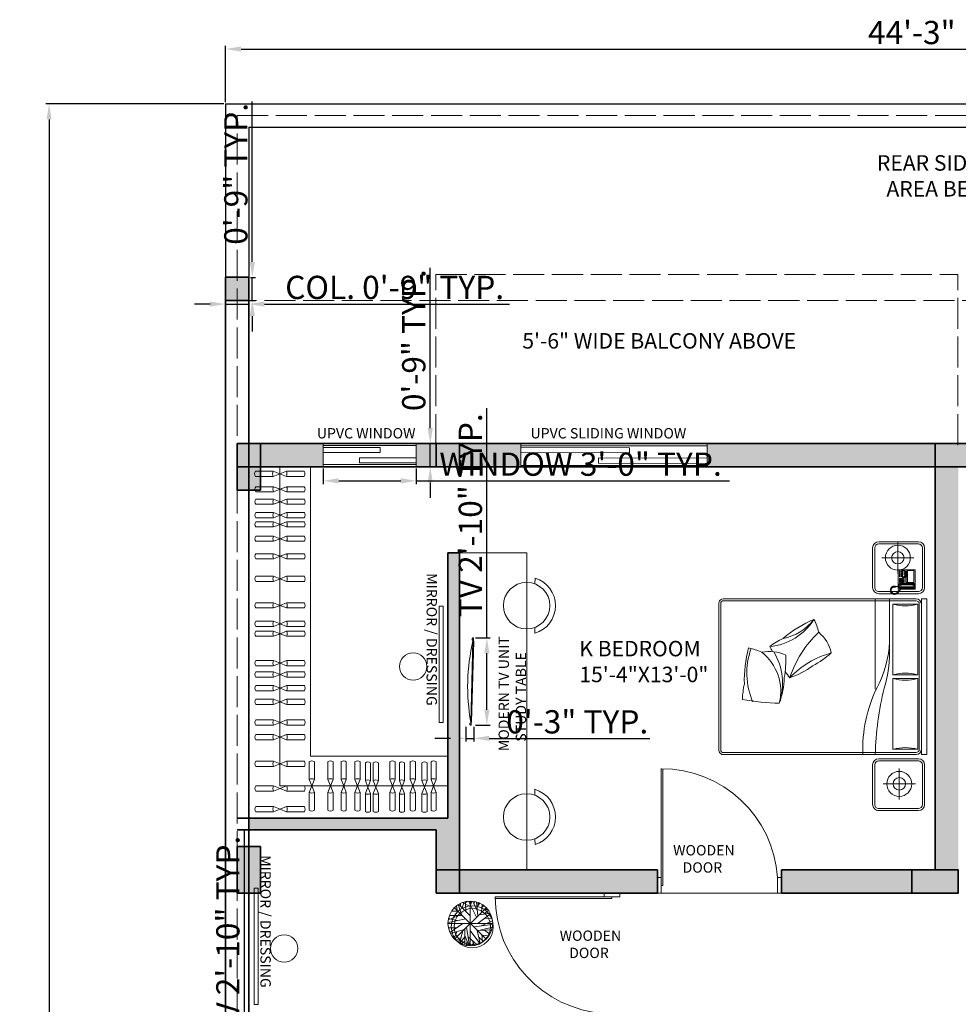
# Model space of a CAD drawing. Units: millimetres. Extents: x 595116 to 630915, y 909473 to 920225.
# Tile 133 of 134: x 630214 to 630577, y 919741 to 920122. Entities that reach past the tile are written whole.
import ezdxf

# ---------------------------------------------------------------- set-up
doc = ezdxf.new("R2010")
doc.units = ezdxf.units.MM
doc.linetypes.add('ACAD_ISO02W100', pattern=[15, 12, -3])
for name, color, linetype, lineweight in [('A-AREA-IDEN', 7, 'Continuous', 20), ('A-EQPM', 8, 'Continuous', 13), ('A-FLOR-BALC', 152, 'Continuous', 18), ('A-FLOR-OVHD', 253, 'ACAD_ISO02W100', 13), ('A-FURN', 32, 'Continuous', 18), ('A-WALL', 1, 'Continuous', 35), ('A-WALL-PATT', 8, 'Continuous', 13), ('C-PROP', 7, 'Continuous', 25), ('C-PROP-REF', 240, 'ACAD_ISO02W100', 13), ('Column', 6, 'Continuous', 35), ('Dimension', 3, 'Continuous', 18), ('Doors', 31, 'Continuous', 20), ('L-PLNT', 85, 'Continuous', 13), ('Text', 7, 'Continuous', 18), ('Windows', 33, 'Continuous', 18)]:
    doc.layers.add(name, color=color, linetype=linetype, lineweight=lineweight)
doc.styles.get("Standard").update_dxf_attribs({"font": 'arial.ttf'})
doc.dimstyles.new('ISO-25', dxfattribs={"dimtxt": 9, "dimasz": 6, "dimexe": 1.25, "dimexo": 0.625, "dimtad": 1, "dimlunit": 4, "dimtxsty": 'Standard', "dimcen": 2.5, "dimadec": 0, "dimazin": 0, "dimtfac": 1, "dimtmove": 0, "dimatfit": 3, "dimfxl": 1, "dimarcsym": 0})

# ---------------------------------------------------------------- blocks, each defined once
blk = doc.blocks.new('KWD')
for points in [[(629753.63, 919957.93), (629752.54, 919957.93), (629752.54, 919953.43), (629753.63, 919953.43)], [(629787.45, 919957.93), (629787.45, 919953.43), (629788.54, 919953.43), (629788.54, 919957.93)]]:
    blk.add_lwpolyline(points, close=True)
blk.add_lwpolyline([(629753.63, 919921.79), (629753.63, 919955.68), (629754.13, 919955.68), (629754.13, 919921.8)])
blk.add_arc((629753.64, 919955.68), 33.88, 269.99, 356.196)
blk = doc.blocks.new('A$C356F0359')
for p, q in [((0.5489, 2), (2.0492, 2)), ((0.5489, 1.9489), (0.5489, 2)), ((2.0492, 1.9489), (2.0492, 2)), ((-0.0002, 1.9201), (-0.0002, 1.5401)), ((0.0198, 1.9201), (0.0198, 1.5401)), ((0.4398, 1.9801), (0.0598, 1.9801)), ((0.4398, 1.9601), (0.0598, 1.9601)), ((0.4798, 1.5401), (0.4798, 1.9201)), ((0.4998, 1.5401), (0.4998, 1.9201)), ((2.0492, 1.9489), (0.5489, 1.9489)), ((0.5489, 1.8977), (0.5489, 0.0512)), ((0.5689, 1.8977), (0.5689, 0.0512)), ((1.998, 1.9289), (0.6001, 1.9289)), ((2.0292, 0.0512), (2.0292, 1.8977)), ((2.0492, 0.0512), (2.0492, 1.8977)), ((2.0883, 1.9201), (2.0883, 1.5401)), ((2.1083, 1.9201), (2.1083, 1.5401)), ((2.5283, 1.9801), (2.1483, 1.9801)), ((2.5283, 1.9601), (2.1483, 1.9601)), ((2.5683, 1.5401), (2.5683, 1.9201)), ((2.5883, 1.5401), (2.5883, 1.9201)), ((0.1539, 1.5681), (0.1539, 1.8777)), ((0.2725, 1.8879), (0.2702, 1.8856)), ((0.2702, 1.8856), (0.2702, 1.7279)), ((0.2725, 1.8879), (0.4531, 1.8879)), ((0.3913, 1.8753), (0.277, 1.8753)), ((0.277, 1.8753), (0.277, 1.8147)), ((0.277, 1.8147), (0.3913, 1.8147)), ((0.3913, 1.8125), (0.2816, 1.8125)), ((0.2816, 1.8125), (0.2816, 1.801)), ((0.2816, 1.801), (0.3913, 1.801)), ((0.2907, 1.8125), (0.2907, 1.801)), ((0.2999, 1.8125), (0.2999, 1.801)), ((0.309, 1.8125), (0.309, 1.801)), ((0.3182, 1.8125), (0.3182, 1.801)), ((0.3273, 1.8125), (0.3273, 1.801)), ((0.3365, 1.8125), (0.3365, 1.801)), ((0.3913, 1.8147), (0.3913, 1.8753)), ((0.3913, 1.801), (0.3913, 1.8125)), ((0.4016, 1.8787), (0.4062, 1.8845)), ((0.4016, 1.7404), (0.4016, 1.8787)), ((0.4062, 1.881), (0.405, 1.8765)), ((0.405, 1.8765), (0.4153, 1.8662)), ((0.405, 1.8765), (0.405, 1.8456)), ((0.405, 1.8456), (0.4073, 1.8399)), ((0.4062, 1.8845), (0.4405, 1.8845)), ((0.4108, 1.8833), (0.4062, 1.881)), ((0.4073, 1.8399), (0.4108, 1.8342)), ((0.4108, 1.8833), (0.4382, 1.8833)), ((0.4165, 1.8685), (0.4108, 1.8833)), ((0.4108, 1.8342), (0.4119, 1.8262)), ((0.4119, 1.8262), (0.4119, 1.8147)), ((0.4119, 1.793), (0.4119, 1.8147)), ((0.4153, 1.8662), (0.4165, 1.8685)), ((0.4153, 1.8147), (0.4153, 1.8662)), ((0.4153, 1.8147), (0.4153, 1.753)), ((0.4325, 1.8685), (0.4165, 1.8685)), ((0.4325, 1.8685), (0.4382, 1.8833)), ((0.4336, 1.8662), (0.4325, 1.8685)), ((0.4439, 1.8765), (0.4336, 1.8662)), ((0.4336, 1.8147), (0.4336, 1.8662)), ((0.4336, 1.8147), (0.4336, 1.753)), ((0.4382, 1.8342), (0.4371, 1.8262)), ((0.4371, 1.8262), (0.4371, 1.8147)), ((0.4371, 1.793), (0.4371, 1.8147)), ((0.4382, 1.8833), (0.4428, 1.881)), ((0.4416, 1.8399), (0.4382, 1.8342)), ((0.4405, 1.8845), (0.4462, 1.8787)), ((0.4439, 1.8456), (0.4416, 1.8399)), ((0.4428, 1.881), (0.4439, 1.8765)), ((0.4439, 1.8765), (0.4439, 1.8456)), ((0.4462, 1.8787), (0.4462, 1.7416)), ((0.4531, 1.8879), (0.4553, 1.8856)), ((0.4553, 1.8856), (0.4553, 1.7279)), ((2.3306, 1.5822), (2.3306, 1.8917)), ((0.3052, 1.7226), (0.0051, 1.7226)), ((0.2702, 1.7279), (0.2725, 1.7256)), ((0.4244, 1.7256), (0.2725, 1.7256)), ((0.277, 1.7885), (0.277, 1.7679)), ((0.3445, 1.7885), (0.277, 1.7885)), ((0.277, 1.7679), (0.3445, 1.7679)), ((0.2782, 1.7622), (0.2782, 1.7576)), ((0.2896, 1.7622), (0.2782, 1.7622)), ((0.2782, 1.7576), (0.2896, 1.7576)), ((0.2782, 1.745), (0.2896, 1.745)), ((0.2782, 1.7382), (0.2782, 1.745)), ((0.2896, 1.7382), (0.2782, 1.7382)), ((0.2885, 1.7862), (0.2885, 1.7827)), ((0.2919, 1.7862), (0.2885, 1.7862)), ((0.2885, 1.7827), (0.2919, 1.7827)), ((0.2919, 1.7736), (0.2885, 1.7736)), ((0.2885, 1.7736), (0.2885, 1.7702)), ((0.2885, 1.7702), (0.2919, 1.7702)), ((0.2896, 1.7576), (0.2896, 1.7622)), ((0.2896, 1.745), (0.2896, 1.7382)), ((0.2919, 1.7827), (0.2919, 1.7862)), ((0.2919, 1.7702), (0.2919, 1.7736)), ((0.2942, 1.7622), (0.2942, 1.7576)), ((0.3056, 1.7622), (0.2942, 1.7622)), ((0.2942, 1.7576), (0.3056, 1.7576)), ((0.2942, 1.745), (0.3056, 1.745)), ((0.2942, 1.7382), (0.2942, 1.745)), ((0.3056, 1.7382), (0.2942, 1.7382)), ((0.3056, 1.7576), (0.3056, 1.7622)), ((0.3056, 1.745), (0.3056, 1.7382)), ((0.3125, 1.7862), (0.309, 1.7862)), ((0.309, 1.7862), (0.309, 1.7827)), ((0.309, 1.7827), (0.3125, 1.7827)), ((0.3125, 1.7736), (0.309, 1.7736)), ((0.309, 1.7736), (0.309, 1.7702)), ((0.309, 1.7702), (0.3125, 1.7702)), ((0.3102, 1.7622), (0.3102, 1.7576)), ((0.3216, 1.7622), (0.3102, 1.7622)), ((0.3102, 1.7576), (0.3216, 1.7576)), ((0.3102, 1.745), (0.3216, 1.745)), ((0.3102, 1.7382), (0.3102, 1.745)), ((0.3216, 1.7382), (0.3102, 1.7382)), ((0.3125, 1.7827), (0.3125, 1.7862)), ((0.3125, 1.7702), (0.3125, 1.7736)), ((0.3216, 1.7576), (0.3216, 1.7622)), ((0.3216, 1.745), (0.3216, 1.7382)), ((0.3376, 1.7622), (0.3262, 1.7622)), ((0.3262, 1.7622), (0.3262, 1.7576)), ((0.3262, 1.7576), (0.3376, 1.7576)), ((0.3262, 1.7382), (0.3262, 1.745)), ((0.3262, 1.745), (0.3376, 1.745)), ((0.3376, 1.7382), (0.3262, 1.7382)), ((0.333, 1.7862), (0.3296, 1.7862)), ((0.3296, 1.7862), (0.3296, 1.7827)), ((0.3296, 1.7827), (0.333, 1.7827)), ((0.333, 1.7736), (0.3296, 1.7736)), ((0.3296, 1.7736), (0.3296, 1.7702)), ((0.3296, 1.7702), (0.333, 1.7702)), ((0.333, 1.7827), (0.333, 1.7862)), ((0.333, 1.7702), (0.333, 1.7736)), ((0.3376, 1.7576), (0.3376, 1.7622)), ((0.3376, 1.745), (0.3376, 1.7382)), ((0.3445, 1.7679), (0.3445, 1.7885)), ((0.3548, 1.7759), (0.3548, 1.7827)), ((0.3548, 1.7827), (0.3639, 1.7827)), ((0.3639, 1.7759), (0.3548, 1.7759)), ((0.3548, 1.7633), (0.3548, 1.7702)), ((0.3548, 1.7702), (0.3639, 1.7702)), ((0.3639, 1.7633), (0.3548, 1.7633)), ((0.3548, 1.7564), (0.3639, 1.7564)), ((0.3548, 1.7496), (0.3548, 1.7564)), ((0.3639, 1.7496), (0.3548, 1.7496)), ((0.3548, 1.737), (0.3548, 1.7439)), ((0.3548, 1.7439), (0.3639, 1.7439)), ((0.3639, 1.737), (0.3548, 1.737)), ((0.3639, 1.7827), (0.3639, 1.7759)), ((0.3639, 1.7702), (0.3639, 1.7633)), ((0.3639, 1.7564), (0.3639, 1.7496)), ((0.3639, 1.7439), (0.3639, 1.737)), ((0.3685, 1.7827), (0.3776, 1.7827)), ((0.3685, 1.7759), (0.3685, 1.7827)), ((0.3776, 1.7759), (0.3685, 1.7759)), ((0.3685, 1.7633), (0.3685, 1.7702)), ((0.3685, 1.7702), (0.3776, 1.7702)), ((0.3776, 1.7633), (0.3685, 1.7633)), ((0.3685, 1.7564), (0.3776, 1.7564)), ((0.3685, 1.7496), (0.3685, 1.7564)), ((0.3776, 1.7496), (0.3685, 1.7496)), ((0.3685, 1.737), (0.3685, 1.7439)), ((0.3685, 1.7439), (0.3776, 1.7439)), ((0.3776, 1.737), (0.3685, 1.737)), ((0.3776, 1.7827), (0.3776, 1.7759)), ((0.3776, 1.7702), (0.3776, 1.7633)), ((0.3776, 1.7564), (0.3776, 1.7496)), ((0.3776, 1.7439), (0.3776, 1.737)), ((0.3822, 1.7759), (0.3822, 1.7827)), ((0.3822, 1.7827), (0.3913, 1.7827)), ((0.3913, 1.7759), (0.3822, 1.7759)), ((0.3822, 1.7633), (0.3822, 1.7702)), ((0.3822, 1.7702), (0.3913, 1.7702)), ((0.3913, 1.7633), (0.3822, 1.7633)), ((0.3822, 1.7576), (0.3913, 1.7576)), ((0.3822, 1.7507), (0.3822, 1.7576)), ((0.3913, 1.7507), (0.3822, 1.7507)), ((0.3822, 1.7439), (0.3913, 1.7439)), ((0.3822, 1.737), (0.3822, 1.7439)), ((0.3913, 1.737), (0.3822, 1.737)), ((0.3913, 1.7827), (0.3913, 1.7759)), ((0.3913, 1.7702), (0.3913, 1.7633)), ((0.3913, 1.7576), (0.3913, 1.7507)), ((0.3913, 1.7439), (0.3913, 1.737)), ((0.4073, 1.7347), (0.4016, 1.7404)), ((0.405, 1.7736), (0.4073, 1.7793)), ((0.405, 1.7427), (0.405, 1.7736)), ((0.405, 1.7427), (0.4153, 1.753)), ((0.4062, 1.7382), (0.405, 1.7427)), ((0.4108, 1.7359), (0.4062, 1.7382)), ((0.4073, 1.7793), (0.4108, 1.785)), ((0.4234, 1.7347), (0.4073, 1.7347)), ((0.4108, 1.785), (0.4119, 1.793)), ((0.4165, 1.7507), (0.4108, 1.7359)), ((0.4108, 1.7359), (0.4234, 1.7359)), ((0.4153, 1.753), (0.4165, 1.7507)), ((0.4325, 1.7507), (0.4165, 1.7507)), ((0.4233, 1.7393), (0.4235, 1.7294)), ((0.4268, 1.7393), (0.4233, 1.7393)), ((0.4235, 1.7294), (0.4263, 1.7179)), ((0.4263, 1.7179), (0.429, 1.707)), ((0.4274, 1.7301), (0.4268, 1.7393)), ((0.427, 1.7359), (0.4382, 1.7359)), ((0.4405, 1.7347), (0.4271, 1.7347)), ((0.429, 1.7227), (0.4274, 1.7301)), ((0.4531, 1.7256), (0.4284, 1.7256)), ((0.429, 1.707), (0.4288, 1.701)), ((0.4318, 1.7119), (0.429, 1.7227)), ((0.4325, 1.7063), (0.4318, 1.7119)), ((0.4323, 1.7003), (0.4325, 1.7063)), ((0.4336, 1.753), (0.4325, 1.7507)), ((0.4325, 1.7507), (0.4382, 1.7359)), ((0.4439, 1.7427), (0.4336, 1.753)), ((0.4382, 1.785), (0.4371, 1.793)), ((0.4416, 1.7793), (0.4382, 1.785)), ((0.4382, 1.7359), (0.4428, 1.7382)), ((0.4462, 1.7416), (0.4405, 1.7347)), ((0.4439, 1.7736), (0.4416, 1.7793)), ((0.4428, 1.7382), (0.4439, 1.7427)), ((0.4439, 1.7427), (0.4439, 1.7736)), ((0.4553, 1.7279), (0.4531, 1.7256)), ((0.4622, 1.7459), (0.4553, 1.7484)), ((0.4553, 1.7439), (0.4604, 1.7425)), ((0.4604, 1.7425), (0.465, 1.7388)), ((0.4654, 1.7427), (0.4622, 1.7459)), ((0.465, 1.7388), (0.4662, 1.7372)), ((0.4678, 1.7405), (0.4654, 1.7427)), ((0.4662, 1.7372), (0.4686, 1.7374)), ((0.4686, 1.7374), (0.4662, 1.735)), ((0.4662, 1.735), (0.4755, 1.7268)), ((0.4721, 1.7421), (0.4678, 1.7405)), ((0.4741, 1.7401), (0.4721, 1.7421)), ((0.4725, 1.7366), (0.4741, 1.7401)), ((0.4753, 1.7388), (0.4725, 1.7366)), ((0.4783, 1.7356), (0.4753, 1.7388)), ((0.4755, 1.7268), (0.4906, 1.7139)), ((0.4759, 1.729), (0.4783, 1.7356)), ((0.4821, 1.7322), (0.4759, 1.729)), ((0.4874, 1.7272), (0.4821, 1.7322)), ((0.4862, 1.7199), (0.4874, 1.7272)), ((0.4914, 1.7231), (0.4862, 1.7199)), ((0.4908, 1.7135), (0.4984, 1.6917)), ((0.4958, 1.7185), (0.4914, 1.7231)), ((0.494, 1.7135), (0.4958, 1.7185)), ((0.501, 1.7142), (0.494, 1.7135)), ((0.4964, 1.7047), (0.5031, 1.7072)), ((0.5031, 1.7072), (0.501, 1.7142)), ((2.4819, 1.7366), (2.1818, 1.7366)), ((0.427, 1.697), (0.4265, 1.6915)), ((0.4265, 1.6915), (0.4332, 1.6903)), ((0.4332, 1.6903), (0.4267, 1.6864)), ((0.4267, 1.6864), (0.4272, 1.6801)), ((0.4295, 1.6996), (0.427, 1.697)), ((0.4272, 1.6801), (0.4346, 1.6794)), ((0.4346, 1.6794), (0.4281, 1.6744)), ((0.4281, 1.6744), (0.4311, 1.669)), ((0.4288, 1.701), (0.4295, 1.6996)), ((0.4311, 1.669), (0.4381, 1.6704)), ((0.4364, 1.6973), (0.4323, 1.7003)), ((0.4381, 1.6704), (0.4348, 1.6639)), ((0.4348, 1.6639), (0.4383, 1.6598)), ((0.4355, 1.6919), (0.4364, 1.6973)), ((0.4367, 1.6774), (0.4355, 1.6919)), ((0.4455, 1.6663), (0.4367, 1.6774)), ((0.4383, 1.6598), (0.4436, 1.6637)), ((0.4436, 1.6637), (0.4427, 1.6575)), ((0.4427, 1.6575), (0.4471, 1.6547)), ((0.4577, 1.6598), (0.4455, 1.6663)), ((0.4471, 1.6547), (0.4526, 1.6593)), ((0.4526, 1.6593), (0.4519, 1.6517)), ((0.4519, 1.6517), (0.4568, 1.6503)), ((0.4568, 1.6503), (0.4598, 1.6565)), ((0.4716, 1.6586), (0.4577, 1.6598)), ((0.4598, 1.6565), (0.4626, 1.6503)), ((0.4626, 1.6503), (0.4665, 1.6498)), ((0.4665, 1.6498), (0.4681, 1.6565)), ((0.4681, 1.6565), (0.4707, 1.6491)), ((0.4707, 1.6491), (0.4751, 1.6503)), ((0.485, 1.6644), (0.4716, 1.6586)), ((0.4751, 1.6503), (0.4753, 1.6565)), ((0.4753, 1.6565), (0.4806, 1.6519)), ((0.4806, 1.6519), (0.4843, 1.6538)), ((0.4843, 1.6538), (0.4836, 1.6607)), ((0.4836, 1.6607), (0.4885, 1.6547)), ((0.4952, 1.6744), (0.485, 1.6644)), ((0.4885, 1.6547), (0.4922, 1.6579)), ((0.4922, 1.6579), (0.4894, 1.6642)), ((0.4894, 1.6642), (0.4959, 1.6614)), ((0.4984, 1.6917), (0.4952, 1.6744)), ((0.4957, 1.6704), (0.5024, 1.6683)), ((0.4989, 1.6642), (0.4957, 1.6704)), ((0.4959, 1.6614), (0.4989, 1.6642)), ((0.5038, 1.7049), (0.4964, 1.7047)), ((0.5042, 1.673), (0.4987, 1.6792)), ((0.4987, 1.6792), (0.5058, 1.679)), ((0.5005, 1.695), (0.5054, 1.6996)), ((0.5068, 1.695), (0.5005, 1.695)), ((0.5008, 1.6871), (0.5079, 1.6892)), ((0.5068, 1.6836), (0.5008, 1.6871)), ((0.5024, 1.6683), (0.5042, 1.673)), ((0.5054, 1.6996), (0.5038, 1.7049)), ((0.5058, 1.679), (0.5068, 1.6836)), ((0.5079, 1.6892), (0.5068, 1.695)), ((0.0598, 1.5001), (0.4398, 1.5001)), ((0.0598, 1.4801), (0.4398, 1.4801)), ((2.1483, 1.5001), (2.5283, 1.5001)), ((2.1483, 1.4801), (2.5283, 1.4801)), ((0.6001, 0.02), (1.998, 0.02)), ((0.6001, 0), (1.998, 0))]:
    blk.add_line(p, q)
at = {"linetype": 'ByBlock'}
for p, q in [((0.6001, 1.9147), (1.282, 1.9147)), ((0.6001, 1.6759), (0.6001, 1.9147)), ((1.282, 1.9147), (1.282, 1.6759)), ((1.3161, 1.9147), (1.998, 1.9147)), ((1.3161, 1.6759), (1.3161, 1.9147)), ((1.998, 1.9147), (1.998, 1.6759)), ((1.0687, 1.6418), (0.5489, 1.6418)), ((1.282, 1.6759), (0.6001, 1.6759)), ((1.998, 1.6759), (1.3161, 1.6759)), ((1.4185, 1.5053), (0.5489, 1.5053))]:
    blk.add_line(p, q, dxfattribs=at)
for centre in [(0.1539, 1.7226), (2.3306, 1.7366)]:
    blk.add_circle(centre, 0.12, dxfattribs=at)
for centre in [(0.1539, 1.7226), (2.3306, 1.7366)]:
    blk.add_circle(centre, 0.06)
for centre, radius, start, end in [((0.0598, 1.9201), 0.06, 90, 180), ((0.0598, 1.9201), 0.04, 90, 180), ((0.4398, 1.9201), 0.06, 0, 90), ((0.4398, 1.9201), 0.04, 0, 90), ((0.6001, 1.8977), 0.0512, 90, 180), ((0.6001, 1.8977), 0.0312, 90, 180), ((1.998, 1.8977), 0.0512, 0, 90), ((1.998, 1.8977), 0.0312, 0, 90), ((2.1483, 1.9201), 0.06, 90, 180), ((2.1483, 1.9201), 0.04, 90, 180), ((2.5283, 1.9201), 0.06, 0, 90), ((2.5283, 1.9201), 0.04, 0, 90), ((0.0598, 1.5401), 0.06, 180, 270), ((0.0598, 1.5401), 0.04, 180, 270), ((0.4398, 1.5401), 0.04, 270, 0), ((0.4398, 1.5401), 0.06, 270, 0), ((2.1483, 1.5401), 0.06, 180, 270), ((2.1483, 1.5401), 0.04, 180, 270), ((2.5283, 1.5401), 0.06, 270, 0), ((2.5283, 1.5401), 0.04, 270, 0), ((1.1471, 0.7332), 0.3575, 102.47819, 140.46254), ((1.9086, 1.3124), 0.8697, 195.33601, 226.41927), ((0.3249, 0.4335), 0.9879, 28.49711, 41.05657), ((0.9965, 0.4273), 0.548, 103.20343, 117.03623), ((1.6529, 1.7059), 1.0798, 223.63057, 251.4288), ((0.4451, 0.4375), 0.5655, 5.33912, 57.68949), ((0.4517, 0.5274), 0.4879, 10.69865, 52.68638), ((1.8195, 1.3719), 1.1652, 203.06416, 220.32086), ((0.5617, 0.4344), 0.7874, 18.35266, 36.68512), ((-0.021, 2.4319), 2.1977, 305.29657, 307.24182), ((1.5949, 0.9312), 0.734, 205.25901, 216.93514), ((1.4135, 0.487), 0.3575, 154.0418, 192.02615), ((1.3641, 0.0041), 0.6085, 71.81005, 120.13512), ((1.44, 0.1186), 0.4774, 76.18494, 142.00166), ((1.1372, -0.3434), 0.9879, 80.06073, 92.62018), ((1.2836, -0.1573), 0.7874, 69.91627, 88.24873), ((-0.6432, 0.628), 2.1977, 349.48843, 358.80544), ((-0.021, 2.4319), 2.1977, 297.92482, 299.3793), ((1.5595, 0.1789), 0.548, 154.76704, 168.59984), ((1.3312, 1.4107), 1.1652, 254.62778, 271.88448), ((1.2647, 0.9578), 0.6885, 250.29361, 293.6414), ((1.5368, 0.9609), 0.734, 256.82263, 268.49876), ((0.5943, 0.0454), 0.0458, 172.75992, 277.24008), ((0.5943, 0.0454), 0.0258, 172.75992, 277.24008), ((2.0038, 0.0454), 0.0458, 262.75992, 7.24008), ((2.0038, 0.0454), 0.0258, 262.75992, 7.24008)]:
    blk.add_arc(centre, radius, start, end)
for centre, radius, start, end in [((0.1906, 1.7953), 0.4265, 343.73979, 16.26021), ((1.6914, 1.7953), 0.4265, 163.73979, 196.26021), ((0.9067, 1.7953), 0.4265, 343.73979, 16.26021), ((2.4075, 1.7953), 0.4265, 163.73979, 196.26021), ((0.9303, 0.657), 0.9853, 61.43285, 88.12613), ((1.0826, 0.5712), 1.0706, 72.19663, 90.74184), ((2.0056, 2.7745), 1.3903, 244.24266, 271.79845), ((2.1368, 4.5996), 3.0955, 256.42012, 268.37887)]:
    blk.add_arc(centre, radius, start, end, dxfattribs=at)
blk = doc.blocks.new('*D129')
at = {"layer": 'Defpoints', "color": 0, "transparency": 16777216}
for p in [(630824.6, 920110.68), (630293.6, 920089.43), (630824.6, 920089.43)]:
    blk.add_point(p, dxfattribs=at)
at = {"layer": 'Dimension', "color": 0, "lineweight": -2, "transparency": 16777216}
for p, q in [((630293.6, 920090.05), (630293.6, 920111.93)), ((630824.6, 920090.05), (630824.6, 920111.93)), ((630299.6, 920110.68), (630818.6, 920110.68))]:
    blk.add_line(p, q, dxfattribs=at)
at = {"layer": 'Dimension', "color": 0, "transparency": 16777216}
for points in [[(630299.6, 920111.68), (630299.6, 920109.68), (630293.6, 920110.68)], [(630818.6, 920111.68), (630818.6, 920109.68), (630824.6, 920110.68)]]:
    blk.add_solid(points, dxfattribs=at)
at = {"layer": 'Dimension', "color": 0, "transparency": 16777216, "insert": (630559.1, 920115.9), "char_height": 9, "attachment_point": 5}
blk.add_mtext('44\'-3"', dxfattribs=at)
blk = doc.blocks.new('TV-PLAN')
for p, q in [((2.04, 32.58), (1.21, 1.19)), ((2.14, 32.58), (1.31, 1.19)), ((2.24, 32.58), (1.41, 1.19)), ((2.34, 32.57), (1.51, 1.18)), ((2.04, 32.58), (2.34, 32.57)), ((2.14, 32.58), (2.14, 33.76)), ((2.19, 32.58), (2.19, 33.76)), ((1.21, 1.19), (1.51, 1.18)), ((1.31, 1.19), (1.31, 0.01)), ((1.36, 1.19), (1.36, 0.01))]:
    blk.add_line(p, q)
for centre, radius, start, end in [((76.63, 14.9), 76.65, 166.662, 190.3006), ((2.09, 33.31), 0.462, 77.1755, 282.8245), ((1.26, 0.46), 0.462, 77.1755, 282.8245)]:
    blk.add_arc(centre, radius, start, end)
blk = doc.blocks.new('WARDROBE-HANGER')
for p, q in [((9.73, 1), (9.73, 1)), ((9.73, 1), (12.27, 0)), ((9.73, 1), (9.73, 1)), ((12.27, 2), (19.15, 2)), ((0.32, 0), (7.19, 0)), ((12.27, 0), (19.15, 0))]:
    blk.add_line(p, q)
for points in [[(7.19, 2), (0.32, 2, 0.315389), (0.32, 0)], [(9.73, 1), (7.19, 2, 0.225748), (7.19, 0), (9.73, 1), (12.27, 2)]]:
    blk.add_lwpolyline(points, format="xyb")
for centre, radius, start, end in [((10.17, 1), 2.33, 334.5576, 25.4424), ((17.71, 1), 1.74, 324.9906, 35.0094)]:
    blk.add_arc(centre, radius, start, end)
blk = doc.blocks.new('POTTED-PLANT')
for p, q in [((14.75, 15.51), (2.6, 3.36)), ((14.75, 3.36), (2.6, 15.51)), ((2.87, 15.88), (3.4, 15.68)), ((3.32, 16.24), (3.58, 14.57)), ((3.96, 16.73), (5.31, 12.84)), ((4.16, 16.82), (8.64, 12.35)), ((4.85, 16.17), (4.88, 17.22)), ((5.49, 15.52), (6.28, 17.77)), ((5.61, 17.51), (8.67, 15.94)), ((6.86, 17.38), (7.52, 18.03)), ((6.89, 14.08), (6.86, 17.93)), ((7.9, 18.06), (11.06, 11.86)), ((9.02, 17.38), (8.46, 18.1)), ((8.67, 18.11), (8.67, 0.76)), ((8.74, 16.47), (9.2, 18.06)), ((11.32, 14.57), (9.46, 18.06)), ((10.09, 16.89), (10.53, 17.9)), ((11.52, 12.26), (11.04, 17.77)), ((11.14, 16.82), (12.03, 17.41)), ((11.24, 15.75), (12.36, 17.28)), ((13.25, 16.79), (13.05, 13.86)), ((13.17, 15.58), (13.86, 16.4)), ((4.01, 12.42), (0.12, 10.79)), ((0.57, 12.45), (5.66, 12.45)), ((1.47, 14.18), (3.93, 14.18)), ((16.53, 13.1), (11.7, 9.48)), ((12.05, 12.81), (16.38, 13.4)), ((13.91, 13.07), (15.74, 14.51)), ((14.04, 14.8), (15.41, 14.87)), ((0, 9.44), (17.35, 9.44)), ((0.04, 9.84), (6.94, 11.18)), ((0.19, 11.28), (3.48, 10.53)), ((0.22, 7.66), (3.4, 7.75)), ((0.78, 5.86), (5.74, 9.45)), ((7.22, 7.98), (8.31, 0.8)), ((10.02, 8.11), (17.3, 9.03)), ((12.49, 6.77), (17.19, 8.01)), ((12.92, 8.47), (17.27, 10.46)), ((14.24, 11.38), (17.09, 11.41)), ((0.98, 5.47), (6.25, 7.04)), ((3.99, 4.75), (1.72, 4.29)), ((3.48, 6.19), (2.31, 3.58)), ((5.1, 3.97), (3.07, 2.83)), ((5.79, 6.51), (4.54, 1.82)), ((6.56, 4.2), (4.67, 1.78)), ((6.53, 7.26), (6.56, 1.1)), ((6.56, 4.78), (8.11, 0.84)), ((7.78, 4.2), (11.26, 1.2)), ((8.67, 6.68), (12.41, 1.65)), ((11.37, 6.74), (12.54, 1.72)), ((11.39, 6.74), (16.97, 6.94)), ((11.98, 4.16), (13.78, 2.43)), ((13.07, 5.08), (13.35, 2.21)), ((13.22, 4.91), (15.85, 4.62)), ((14.19, 6.81), (16.25, 5.24)), ((4.88, 3.09), (3.65, 2.4)), ((6.56, 2.6), (5.05, 1.59)), ((5.56, 2.86), (5.79, 1.33)), ((7.45, 2.57), (7.01, 0.97)), ((7.75, 1.82), (7.32, 0.93)), ((9.89, 1.75), (9.23, 0.84)), ((9.53, 2.7), (10.2, 0.97)), ((12.26, 2.96), (12, 1.49))]:
    blk.add_line(p, q)
for centre, radius in [((8.67, 9.44), 8.67), ((9.43, 8.14), 8.14), ((9.43, 8.14), 7.03)]:
    blk.add_circle(centre, radius)
blk = doc.blocks.new('WIN-UPVC-3FT')
for p, q in [((0, 0), (0, 9)), ((0, 9), (36, 9)), ((36, 0), (36, 9)), ((0, 7.5), (22, 7.5)), ((0, 5.5), (22, 5.5)), ((22, 7.5), (22, 5.5)), ((14, 3.5), (36, 3.5)), ((14, 3.5), (14, 1.5)), ((14, 1.5), (36, 1.5)), ((0, 0), (36, 0))]:
    blk.add_line(p, q)
blk.add_lwpolyline([(0, 8.25), (36, 8.25), (36, 0.89), (0, 0.89)], close=True)
blk = doc.blocks.new('WIN-SLIDING-6FT')
for p, q in [((0, 0), (0, 9)), ((0, 9), (72, 9)), ((72, 0), (72, 9)), ((0, 5.5), (42, 5.41)), ((0.01, 7.5), (42, 7.41)), ((42, 7.41), (42, 5.41)), ((30, 3.44), (72, 3.35)), ((30, 3.44), (30, 1.44)), ((30, 1.44), (71.99, 1.35)), ((0, 0), (72, 0))]:
    blk.add_line(p, q)
blk.add_lwpolyline([(0, 8.12), (72, 8.12), (72, 0.59), (0, 0.59)], close=True)
blk = doc.blocks.new('CHAIR-ROUND')
for p, q in [((12.11, 21.41), (12.12, 19.12)), ((12.2, 2.29), (12.22, 0))]:
    blk.add_line(p, q)
blk.add_circle((8.99, 10.69), 8.99)
blk.add_arc((8.99, 10.69), 11.16, 286.7943, 73.7898)
blk = doc.blocks.new('COLUMN-SQUARE-9IN')
h = blk.add_hatch(color=256)
h.dxf.hatch_style = 1
h.paths.add_polyline_path([(9, 9), (0, 9), (0, 0), (9, 0)])
blk.add_lwpolyline([(0, 9), (9, 9), (9, 0), (0, 0)], close=True)
blk = doc.blocks.new('COLUMN-RECT-18X9')
h = blk.add_hatch(color=256)
h.dxf.hatch_style = 1
h.paths.add_polyline_path([(18, 9), (0, 9), (0, 0), (18, 0)])
blk.add_lwpolyline([(0, 9), (18, 9), (18, 0), (0, 0)], close=True)
blk = doc.blocks.new('COLUMN-RECT-9X18')
h = blk.add_hatch(color=256)
h.dxf.hatch_style = 1
h.paths.add_polyline_path([(9, 18), (0, 18), (0, 0), (9, 0)])
blk.add_lwpolyline([(0, 18), (9, 18), (9, 0), (0, 0)], close=True)
blk = doc.blocks.new('*D156')
at = {"layer": 'Defpoints', "color": 0, "transparency": 16777216}
for p in [(630293.6, 920013.3), (630302.6, 920013.3), (630302.6, 920011.95)]:
    blk.add_point(p, dxfattribs=at)
at = {"layer": 'Dimension', "color": 0, "lineweight": -2, "transparency": 16777216}
for p, q in [((630293.6, 920012.68), (630293.6, 920010.7)), ((630302.6, 920012.68), (630302.6, 920010.7)), ((630287.6, 920011.95), (630281.6, 920011.95)), ((630293.6, 920011.95), (630302.6, 920011.95)), ((630308.6, 920011.95), (630403.44, 920011.95))]:
    blk.add_line(p, q, dxfattribs=at)
at = {"layer": 'Dimension', "color": 0, "transparency": 16777216}
for points in [[(630287.6, 920012.95), (630287.6, 920010.95), (630293.6, 920011.95)], [(630308.6, 920012.95), (630308.6, 920010.95), (630302.6, 920011.95)]]:
    blk.add_solid(points, dxfattribs=at)
at = {"layer": 'Dimension', "color": 0, "transparency": 16777216, "insert": (630359.02, 920017.23), "char_height": 9, "attachment_point": 5}
blk.add_mtext('COL. 0\'-9" TYP.', dxfattribs=at)
blk = doc.blocks.new('*D157')
at = {"layer": 'Defpoints', "color": 0, "transparency": 16777216}
for p in [(630302.6, 920022.3), (630303.95, 920022.3), (630302.6, 920013.3)]:
    blk.add_point(p, dxfattribs=at)
at = {"layer": 'Dimension', "color": 0, "lineweight": -2, "transparency": 16777216}
for p, q in [((630303.95, 920028.3), (630303.95, 920090.41)), ((630303.22, 920022.3), (630305.2, 920022.3)), ((630303.95, 920013.3), (630303.95, 920022.3)), ((630303.22, 920013.3), (630305.2, 920013.3)), ((630303.95, 920007.3), (630303.95, 920001.3))]:
    blk.add_line(p, q, dxfattribs=at)
at = {"layer": 'Dimension', "color": 0, "transparency": 16777216}
for points in [[(630302.95, 920028.3), (630304.95, 920028.3), (630303.95, 920022.3)], [(630302.95, 920007.3), (630304.95, 920007.3), (630303.95, 920013.3)]]:
    blk.add_solid(points, dxfattribs=at)
at = {"layer": 'Dimension', "color": 0, "transparency": 16777216, "insert": (630298.73, 920062.36), "char_height": 9, "attachment_point": 5, "rotation": 90}
blk.add_mtext('0\'-9" TYP.', dxfattribs=at)
blk = doc.blocks.new('*D174')
at = {"layer": 'Defpoints', "color": 0, "transparency": 16777216}
for p in [(630389.62, 919882.75), (630394.69, 919882.75), (630389.62, 919848.92)]:
    blk.add_point(p, dxfattribs=at)
at = {"layer": 'Dimension', "color": 0, "lineweight": -2, "transparency": 16777216}
for p, q in [((630394.69, 919882.75), (630394.69, 919971.64)), ((630390.24, 919882.75), (630395.94, 919882.75)), ((630394.69, 919854.92), (630394.69, 919876.75)), ((630390.24, 919848.92), (630395.94, 919848.92))]:
    blk.add_line(p, q, dxfattribs=at)
at = {"layer": 'Dimension', "color": 0, "transparency": 16777216}
for points in [[(630393.69, 919876.75), (630395.69, 919876.75), (630394.69, 919882.75)], [(630393.69, 919854.92), (630395.69, 919854.92), (630394.69, 919848.92)]]:
    blk.add_solid(points, dxfattribs=at)
at = {"layer": 'Dimension', "color": 0, "transparency": 16777216, "insert": (630389.47, 919930.19), "char_height": 9, "attachment_point": 5, "rotation": 90}
blk.add_mtext('TV 2\'-10" TYP.', dxfattribs=at)
blk = doc.blocks.new('*D175')
at = {"layer": 'Defpoints', "color": 0, "transparency": 16777216}
for p in [(630386.59, 919848.92), (630389.62, 919848.92), (630389.62, 919843.84)]:
    blk.add_point(p, dxfattribs=at)
at = {"layer": 'Dimension', "color": 0, "lineweight": -2, "transparency": 16777216}
for p, q in [((630386.59, 919848.29), (630386.59, 919842.59)), ((630389.62, 919848.29), (630389.62, 919842.59)), ((630380.59, 919843.84), (630374.59, 919843.84)), ((630386.59, 919843.84), (630389.62, 919843.84)), ((630395.62, 919843.84), (630457.73, 919843.84))]:
    blk.add_line(p, q, dxfattribs=at)
at = {"layer": 'Dimension', "color": 0, "transparency": 16777216}
for points in [[(630380.59, 919844.84), (630380.59, 919842.84), (630386.59, 919843.84)], [(630395.62, 919844.84), (630395.62, 919842.84), (630389.62, 919843.84)]]:
    blk.add_solid(points, dxfattribs=at)
at = {"layer": 'Dimension', "color": 0, "transparency": 16777216, "insert": (630429.67, 919849.06), "char_height": 9, "attachment_point": 5}
blk.add_mtext('0\'-3" TYP.', dxfattribs=at)
blk = doc.blocks.new('*D176')
at = {"layer": 'Defpoints', "color": 0, "transparency": 16777216}
for p in [(630300.87, 919719.25), (630305.94, 919719.25), (630305.94, 919685.42)]:
    blk.add_point(p, dxfattribs=at)
at = {"layer": 'Dimension', "color": 0, "lineweight": -2, "transparency": 16777216}
for p, q in [((630300.87, 919719.25), (630300.87, 919808.14)), ((630305.32, 919719.25), (630299.62, 919719.25)), ((630300.87, 919691.42), (630300.87, 919713.25)), ((630305.32, 919685.42), (630299.62, 919685.42))]:
    blk.add_line(p, q, dxfattribs=at)
at = {"layer": 'Dimension', "color": 0, "transparency": 16777216}
for points in [[(630299.87, 919713.25), (630301.87, 919713.25), (630300.87, 919719.25)], [(630299.87, 919691.42), (630301.87, 919691.42), (630300.87, 919685.42)]]:
    blk.add_solid(points, dxfattribs=at)
at = {"layer": 'Dimension', "color": 0, "transparency": 16777216, "insert": (630295.65, 919766.69), "char_height": 9, "attachment_point": 5, "rotation": 90}
blk.add_mtext('TV 2\'-10" TYP.', dxfattribs=at)
blk = doc.blocks.new('*D177')
at = {"layer": 'Defpoints', "color": 0, "transparency": 16777216}
for p in [(630308.97, 919724.32), (630305.94, 919719.25), (630308.97, 919719.25)]:
    blk.add_point(p, dxfattribs=at)
at = {"layer": 'Dimension', "color": 0, "lineweight": -2, "transparency": 16777216}
for p, q in [((630299.94, 919724.32), (630293.94, 919724.32)), ((630305.94, 919719.87), (630305.94, 919725.57)), ((630305.94, 919724.32), (630308.97, 919724.32)), ((630308.97, 919719.87), (630308.97, 919725.57)), ((630314.97, 919724.32), (630377.08, 919724.32))]:
    blk.add_line(p, q, dxfattribs=at)
at = {"layer": 'Dimension', "color": 0, "transparency": 16777216}
for points in [[(630299.94, 919725.32), (630299.94, 919723.32), (630305.94, 919724.32)], [(630314.97, 919725.32), (630314.97, 919723.32), (630308.97, 919724.32)]]:
    blk.add_solid(points, dxfattribs=at)
at = {"layer": 'Dimension', "color": 0, "transparency": 16777216, "insert": (630349.02, 919729.55), "char_height": 9, "attachment_point": 5}
blk.add_mtext('0\'-3" TYP.', dxfattribs=at)
blk = doc.blocks.new('*D190')
at = {"layer": 'Defpoints', "color": 0, "transparency": 16777216}
for p in [(630331.39, 919948.93), (630367.39, 919948.93), (630367.39, 919943.53)]:
    blk.add_point(p, dxfattribs=at)
at = {"layer": 'Dimension', "color": 0, "lineweight": -2, "transparency": 16777216}
for p, q in [((630331.39, 919948.3), (630331.39, 919942.28)), ((630367.39, 919948.3), (630367.39, 919942.28)), ((630337.39, 919943.53), (630361.39, 919943.53)), ((630367.39, 919943.53), (630488.53, 919943.53))]:
    blk.add_line(p, q, dxfattribs=at)
at = {"layer": 'Dimension', "color": 0, "transparency": 16777216}
for points in [[(630337.39, 919944.53), (630337.39, 919942.53), (630331.39, 919943.53)], [(630361.39, 919944.53), (630361.39, 919942.53), (630367.39, 919943.53)]]:
    blk.add_solid(points, dxfattribs=at)
at = {"layer": 'Dimension', "color": 0, "transparency": 16777216, "insert": (630430.96, 919948.81), "char_height": 9, "attachment_point": 5}
blk.add_mtext('WINDOW 3\'-0" TYP.', dxfattribs=at)
blk = doc.blocks.new('*D191')
at = {"layer": 'Defpoints', "color": 0, "transparency": 16777216}
for p in [(630367.39, 919957.93), (630372.79, 919957.93), (630367.39, 919948.93)]:
    blk.add_point(p, dxfattribs=at)
at = {"layer": 'Dimension', "color": 0, "lineweight": -2, "transparency": 16777216}
for p, q in [((630372.79, 919963.93), (630372.79, 920026.04)), ((630368.02, 919957.93), (630374.04, 919957.93)), ((630372.79, 919948.93), (630372.79, 919957.93)), ((630368.02, 919948.93), (630374.04, 919948.93)), ((630372.79, 919942.93), (630372.79, 919936.93))]:
    blk.add_line(p, q, dxfattribs=at)
at = {"layer": 'Dimension', "color": 0, "transparency": 16777216}
for points in [[(630371.79, 919963.93), (630373.79, 919963.93), (630372.79, 919957.93)], [(630371.79, 919942.93), (630373.79, 919942.93), (630372.79, 919948.93)]]:
    blk.add_solid(points, dxfattribs=at)
at = {"layer": 'Dimension', "color": 0, "transparency": 16777216, "insert": (630367.57, 919997.98), "char_height": 9, "attachment_point": 5, "rotation": 90}
blk.add_mtext('0\'-9" TYP.', dxfattribs=at)
blk = doc.blocks.new('*D214')
at = {"layer": 'Defpoints', "color": 0, "transparency": 16777216}
for p in [(630293.6, 920089.43), (630225.3, 919146.43), (630293.6, 919146.43)]:
    blk.add_point(p, dxfattribs=at)
at = {"layer": 'Dimension', "color": 0, "lineweight": -2, "transparency": 16777216}
for p, q in [((630292.97, 920089.43), (630224.05, 920089.43)), ((630225.3, 920083.43), (630225.3, 919152.43)), ((630292.97, 919146.43), (630224.05, 919146.43))]:
    blk.add_line(p, q, dxfattribs=at)
at = {"layer": 'Dimension', "color": 0, "transparency": 16777216}
for points in [[(630224.3, 920083.43), (630226.3, 920083.43), (630225.3, 920089.43)], [(630224.3, 919152.43), (630226.3, 919152.43), (630225.3, 919146.43)]]:
    blk.add_solid(points, dxfattribs=at)
at = {"layer": 'Dimension', "color": 0, "transparency": 16777216, "insert": (630220.08, 919617.93), "char_height": 9, "attachment_point": 5, "rotation": 90}
blk.add_mtext('78\'-7"', dxfattribs=at)

msp = doc.modelspace()

# ---------------------------------------------------------------- hatches: boundary and pattern name
at = {"layer": 'A-WALL-PATT'}
h = msp.add_hatch(color=256, dxfattribs=at)
h.dxf.hatch_style = 1
h.paths.add_polyline_path([(630331.391, 919957.928), (630307.096, 919957.928), (630307.096, 919948.928), (630331.391, 919948.928)])
h = msp.add_hatch(color=256, dxfattribs=at)
h.dxf.hatch_style = 1
h.paths.add_polyline_path([(630375.096, 919957.928), (630367.391, 919957.928), (630367.391, 919948.928), (630375.096, 919948.928)])
h = msp.add_hatch(color=256, dxfattribs=at)
h.dxf.hatch_style = 1
h.paths.add_polyline_path([(630407.891, 919957.928), (630384.096, 919957.928), (630384.096, 919948.928), (630407.891, 919948.928)])
h = msp.add_hatch(color=256, dxfattribs=at)
h.dxf.hatch_style = 1
h.paths.add_polyline_path([(630568.096, 919957.928), (630479.891, 919957.928), (630479.891, 919948.928), (630568.096, 919948.928)])
h = msp.add_hatch(color=256, dxfattribs=at)
h.dxf.hatch_style = 1
h.paths.add_polyline_path([(630577.096, 919948.928), (630568.096, 919948.928), (630568.096, 919792.928), (630577.096, 919792.928)])
h = msp.add_hatch(color=256, dxfattribs=at)
h.dxf.hatch_style = 1
h.paths.add_polyline_path([(630384.096, 919915.675), (630379.596, 919915.675), (630379.596, 919812.928), (630302.596, 919812.928), (630302.596, 919808.428), (630375.096, 919808.428), (630375.096, 919792.928), (630384.096, 919792.928)])
h = msp.add_hatch(color=256, dxfattribs=at)
h.dxf.hatch_style = 1
h.paths.add_polyline_path([(630460.656, 919792.928), (630384.096, 919792.928), (630384.096, 919783.928), (630460.656, 919783.928)])
h = msp.add_hatch(color=256, dxfattribs=at)
h.dxf.hatch_style = 1
h.paths.add_polyline_path([(630559.096, 919792.928), (630508.656, 919792.928), (630508.656, 919783.928), (630559.096, 919783.928)])

# ---------------------------------------------------------------- linework, layer by layer
at = {"layer": 'A-FLOR-BALC'}
msp.add_line((630293.596, 920022.301), (630302.596, 920022.301), dxfattribs=at)
at = {"layer": 'A-FLOR-OVHD'}
for p, q in [((630374.891, 919957.393), (630374.891, 920023.393)), ((630374.891, 920023.393), (630576.891, 920023.393)), ((630576.891, 919957.393), (630576.891, 920023.393)), ((630815.596, 920013.301), (630293.596, 920013.301))]:
    msp.add_line(p, q, dxfattribs=at)
at = {"layer": 'A-FURN'}
for p, q in [((630314.561, 919948.928), (630314.561, 919825.399)), ((630326.418, 919836.963), (630326.418, 919948.928)), ((630384.096, 919915.675), (630410.096, 919915.675)), ((630410.096, 919915.675), (630410.096, 919792.928)), ((630326.418, 919836.963), (630379.596, 919836.963)), ((630314.561, 919825.399), (630379.596, 919825.399))]:
    msp.add_line(p, q, dxfattribs=at)
for points in [[(630376.212, 919895.019), (630377.805, 919895.019), (630377.805, 919850.001), (630376.212, 919850.001)], [(630306.233, 919785.867), (630304.64, 919785.867), (630304.64, 919740.848), (630306.233, 919740.848)]]:
    msp.add_lwpolyline(points, close=True, dxfattribs=at)
for centre in [(630366.169, 919871.649), (630316.276, 919762.496)]:
    msp.add_circle(centre, 5.273, dxfattribs=at)
at = {"layer": 'A-WALL'}
for p, q in [((630302.596, 919516.015), (630302.596, 920022.301)), ((630298.096, 919957.928), (630734.596, 919957.928)), ((630298.096, 919948.928), (630568.096, 919948.928)), ((630568.096, 919948.928), (630568.096, 919792.928)), ((630379.596, 919915.675), (630379.596, 919812.928)), ((630379.596, 919915.675), (630384.096, 919915.675)), ((630384.096, 919915.675), (630384.096, 919792.928)), ((630298.096, 919812.928), (630379.596, 919812.928)), ((630298.096, 919808.428), (630375.096, 919808.428)), ((630375.096, 919808.428), (630375.096, 919783.928)), ((630384.096, 919792.928), (630460.656, 919792.928)), ((630460.656, 919792.928), (630460.656, 919783.928)), ((630508.656, 919792.928), (630508.656, 919783.928)), ((630508.656, 919792.928), (630568.096, 919792.928)), ((630375.096, 919783.928), (630460.656, 919783.928)), ((630508.656, 919783.928), (630577.096, 919783.928))]:
    msp.add_line(p, q, dxfattribs=at)
msp.add_lwpolyline([(630293.596, 919516.015), (630293.596, 920022.301)], dxfattribs=at)
at = {"layer": 'C-PROP'}
for p, q in [((630293.596, 920089.428), (630293.596, 920022.301)), ((630302.596, 920080.428), (630815.596, 920080.428)), ((630302.596, 920080.428), (630302.596, 920022.301))]:
    msp.add_line(p, q, dxfattribs=at)
msp.add_lwpolyline([(630293.596, 920089.428), (630824.596, 920089.428)], dxfattribs=at)
at = {"layer": 'C-PROP-REF'}
for p, q in [((630298.096, 920084.928), (630820.096, 920084.928)), ((630298.096, 919150.928), (630298.096, 920084.928))]:
    msp.add_line(p, q, dxfattribs=at)
at = {"layer": 'Doors'}
msp.add_line((630462.114, 919783.928), (630507.199, 919783.928), dxfattribs=at)
at = {"layer": 'Windows'}
for p, q in [((630331.391, 919957.928), (630331.391, 919948.928)), ((630367.391, 919957.928), (630367.391, 919948.928)), ((630407.891, 919957.928), (630407.891, 919948.928)), ((630479.891, 919957.928), (630479.891, 919948.928))]:
    msp.add_line(p, q, dxfattribs=at)

# ---------------------------------------------------------------- block references
at = {"layer": 'A-EQPM'}
msp.add_blockref('TV-PLAN', (630387.275, 919848.948), dxfattribs=at)
at = {"layer": 'A-FURN'}
for name, p in [('WARDROBE-HANGER', (630304.843, 919945.224)), ('WARDROBE-HANGER', (630304.934, 919939.256)), ('WARDROBE-HANGER', (630304.941, 919934.427)), ('WARDROBE-HANGER', (630304.941, 919929.249)), ('WARDROBE-HANGER', (630304.941, 919925.668)), ('WARDROBE-HANGER', (630304.941, 919920.108)), ('WARDROBE-HANGER', (630304.941, 919913.305)), ('WARDROBE-HANGER', (630304.941, 919904.611)), ('WARDROBE-HANGER', (630304.941, 919894.313)), ('WARDROBE-HANGER', (630304.941, 919887.148)), ('WARDROBE-HANGER', (630304.941, 919883.355)), ('WARDROBE-HANGER', (630304.934, 919871.928)), ('WARDROBE-HANGER', (630304.941, 919867.527)), ('WARDROBE-HANGER', (630304.941, 919862.233)), ('WARDROBE-HANGER', (630304.941, 919856.965)), ('WARDROBE-HANGER', (630304.941, 919848.957)), ('WARDROBE-HANGER', (630304.941, 919843.267)), ('WARDROBE-HANGER', (630304.941, 919832.942)), ('WARDROBE-HANGER', (630304.941, 919823.414)), ('CHAIR-ROUND', (630401.106, 919802.696)), ('WARDROBE-HANGER', (630304.941, 919815.407))]:
    msp.add_blockref(name, p, dxfattribs=at)
at = {"layer": 'A-FURN', "xscale": 40.21338437233606, "yscale": 40.21338437233606, "zscale": 40.21338437233606, "rotation": 270}
msp.add_blockref('A$C356F0359', (630484.437, 919919.932), dxfattribs=at)
at = {"layer": 'A-FURN', "extrusion": (0, 0, -1), "zscale": -1, "rotation": 180}
msp.add_blockref('CHAIR-ROUND', (-630401.106, 919905.907), dxfattribs=at)
at = {"layer": 'A-FURN', "rotation": 90}
for p in [(630327.982, 919815.672), (630335.184, 919815.672), (630340.296, 919815.672), (630345.651, 919815.672), (630349.687, 919815.236), (630352.745, 919815.233), (630359.17, 919815.672), (630362.843, 919815.236), (630367.067, 919815.672), (630371.562, 919815.236), (630375.098, 919815.672)]:
    msp.add_blockref('WARDROBE-HANGER', p, dxfattribs=at)
at = {"layer": 'Column'}
for name, p in [('COLUMN-SQUARE-9IN', (630293.596, 920013.301)), ('COLUMN-RECT-9X18', (630298.096, 919939.928)), ('COLUMN-SQUARE-9IN', (630375.096, 919948.928)), ('COLUMN-RECT-18X9', (630568.096, 919948.928)), ('COLUMN-RECT-9X18', (630298.096, 919783.928)), ('COLUMN-SQUARE-9IN', (630375.096, 919783.928)), ('COLUMN-RECT-18X9', (630559.096, 919783.928))]:
    msp.add_blockref(name, p, dxfattribs=at)
at = {"layer": 'Doors', "yscale": 1.333333333333333, "zscale": 1.333333333333333}
for p, xscale, rotation in [((-209209.398, 2146394.498), -1.333333333333333, 180), ((-596164.474, 1759453.982), 1.333333333333333, 270)]:
    msp.add_blockref('KWD', p, dxfattribs=dict(at, xscale=xscale, rotation=rotation))
at = {"layer": 'L-PLNT'}
msp.add_blockref('POTTED-PLANT', (630379.625, 919762.76), dxfattribs=at)
at = {"layer": 'Windows'}
for name, p in [('WIN-UPVC-3FT', (630331.391, 919948.928)), ('WIN-SLIDING-6FT', (630407.891, 919948.928))]:
    msp.add_blockref(name, p, dxfattribs=at)

# ---------------------------------------------------------------- texts
at = {"layer": 'A-AREA-IDEN', "char_height": 6, "attachment_point": 1}
for s, width, insert in [('{REAR SIDE OPEN\\P  AREA BELOW}', 125.26422, (630545.614, 920069.59)), ('{K BEDROOM \\P15\'-4"X13\'-0"}', 83.57324, (630430.462, 919881.567))]:
    msp.add_mtext_dynamic_manual_height_columns(s, width=width, gutter_width=12.5, heights=[0], dxfattribs=dict(at, insert=insert))
at = {"layer": 'Text', "attachment_point": 1}
for s, width, insert, char_height in [('{5\'-6" WIDE BALCONY ABOVE}', 125.26422, (630408.41, 920000.716), 6), ('{ UPVC WINDOW}', 61.33456, (630327.69, 919963.938), 4), ('{ UPVC SLIDING WINDOW}', 72.55106, (630410.358, 919963.938), 4), ('{     WOODEN\\P        DOOR}', 61.33456, (630460.656, 919802.518), 4), ('{     WOODEN\\P        DOOR}', 61.33456, (630416.759, 919769.451), 4)]:
    msp.add_mtext_dynamic_manual_height_columns(s, width=width, gutter_width=12.5, heights=[0], dxfattribs=dict(at, insert=insert, char_height=char_height))
at = {"layer": 'Text', "char_height": 4}
for s, insert, attachment_point, rotation in [('{    MIRROR / DRESSING}', (630375.363, 919912.653), 1, 270), ('{     MODERN TV UNIT\\P        STUDY TABLE}', (630399.222, 919832.765), 1, 90), ('{    MIRROR / DRESSING}', (630307.082, 919803.5), 7, 270)]:
    msp.add_mtext_dynamic_manual_height_columns(s, width=72.55106, gutter_width=12.5, heights=[0], dxfattribs=dict(at, insert=insert, attachment_point=attachment_point, rotation=rotation))

# ---------------------------------------------------------------- dimensions: what is measured, and where the dimension line sits
at = {"layer": 'Dimension'}
dim = msp.add_linear_dim(base=(630824.596, 920110.681), p1=(630293.596, 920089.428), p2=(630824.596, 920089.428), dimstyle='ISO-25', override={"dimclrd": 0, "dimclre": 0, "dimclrt": 0}, dxfattribs=at)
dim.commit()
dim.dimension.update_dxf_attribs({"geometry": '*D129', "text_midpoint": (630559.096, 920115.904)})
dim = msp.add_linear_dim(base=(630225.296, 919146.428), p1=(630293.596, 920089.428), p2=(630293.596, 919146.428), angle=90, dimstyle='ISO-25', override={"dimdec": 1, "dimlfac": 1, "dimrnd": 0, "dimzin": 1, "dimdsep": 46, "dimlunit": 4, "dimfrac": 2}, dxfattribs=at)
dim.commit()
dim.dimension.update_dxf_attribs({"geometry": '*D214', "text_midpoint": (630220.076, 919617.928)})
for base, p1, p2, text, picture, middle in [((630303.946, 920022.301), (630302.596, 920013.301), (630302.596, 920022.301), '<> TYP.', '*D157', (630298.726, 920062.355)), ((630372.791, 919957.928), (630367.391, 919948.928), (630367.391, 919957.928), '<> TYP.', '*D191', (630367.57, 919997.982)), ((630394.693, 919882.747), (630389.619, 919848.916), (630389.619, 919882.747), 'TV <> TYP.', '*D174', (630389.473, 919930.192)), ((630300.869, 919719.247), (630305.943, 919685.416), (630305.943, 919719.247), 'TV <> TYP.', '*D176', (630295.649, 919766.692))]:
    dim = msp.add_linear_dim(base=base, p1=p1, p2=p2, angle=90, text=text, dimstyle='ISO-25', override={"dimdec": 1, "dimlfac": 1, "dimrnd": 0, "dimzin": 1, "dimdsep": 46, "dimlunit": 4, "dimfrac": 2}, dxfattribs=at)
    dim.commit()
    dim.dimension.update_dxf_attribs({"geometry": picture, "text_midpoint": middle})
for base, p1, p2, text, picture, middle in [((630302.596, 920011.951), (630293.596, 920013.301), (630302.596, 920013.301), 'COL. <> TYP.', '*D156', (630359.018, 920017.232)), ((630367.391, 919943.528), (630331.391, 919948.928), (630367.391, 919948.928), 'WINDOW <> TYP.', '*D190', (630430.959, 919948.812)), ((630389.619, 919843.842), (630386.595, 919848.916), (630389.619, 919848.916), '<> TYP.', '*D175', (630429.674, 919849.065)), ((630308.967, 919724.322), (630305.943, 919719.247), (630308.967, 919719.247), '<> TYP.', '*D177', (630349.022, 919729.545))]:
    dim = msp.add_linear_dim(base=base, p1=p1, p2=p2, text=text, dimstyle='ISO-25', override={"dimdec": 1, "dimlfac": 1, "dimrnd": 0, "dimzin": 1, "dimdsep": 46, "dimlunit": 4, "dimfrac": 2}, dxfattribs=at)
    dim.commit()
    dim.dimension.update_dxf_attribs({"geometry": picture, "text_midpoint": middle})

doc.saveas('drawing.dxf')
